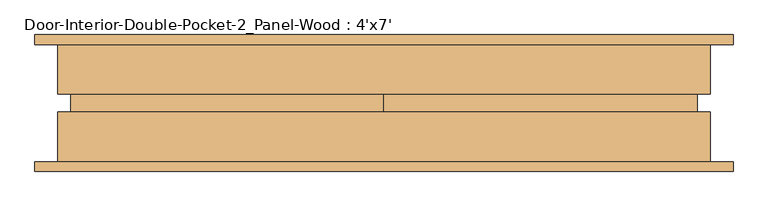
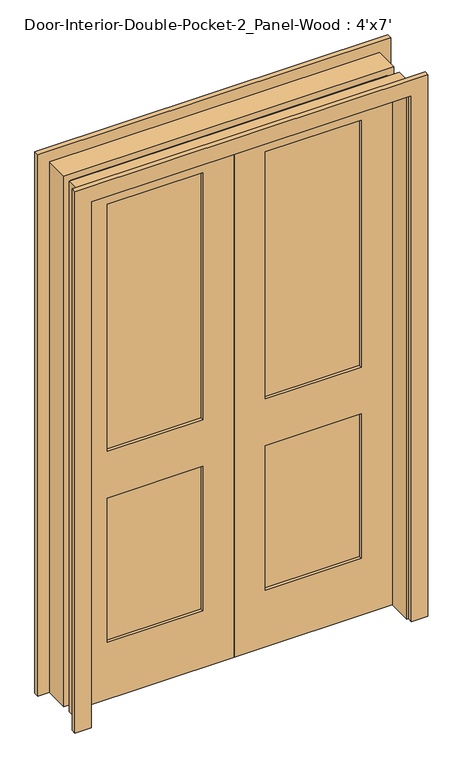
"""IFC4 building model written with IfcOpenShell, lengths in millimetres: door geometry, Door-Interior-Double-Pocket-2_Panel-Wood : 4'x7'."""

from ifc_helpers import new_model, si_unit, frame, origin, place, context, project, spatial, polyline, outline, extrude, source, transform, mapped, element, save


def door_interior_double_pocket_2_panel_wood_4_x7_3a565322(model_context):
    return source(origin(), model_context, "Body", "SweptSolid", [
        extrude(outline(polyline([(0.0, 615.95), (0.0, 679.45), (2203.45, 679.45), (2203.45, -679.45), (0.0, -679.45), (0.0, -615.95), (2139.95, -615.95), (2139.95, 615.95), (0.0, 615.95)])), frame((0.0, 114.3, 0.0), z_axis=(0.0, 1.0, 0.0), x_axis=(0.0, 0.0, 1.0)), (0.0, 0.0, 1.0), 19.05),
        extrude(outline(polyline([(0.0, 615.95), (0.0, 679.45), (2203.45, 679.45), (2203.45, -679.45), (0.0, -679.45), (0.0, -615.95), (2139.95, -615.95), (2139.95, 615.95), (0.0, 615.95)])), frame((0.0, -133.35, 0.0), z_axis=(0.0, 1.0, 0.0), x_axis=(0.0, 0.0, 1.0)), (0.0, 0.0, 1.0), 19.05),
        extrude(outline(polyline([(2133.6, 0.0), (0.0, 0.0), (0.0, 609.6), (2133.6, 609.6), (2133.6, 0.0)]), holes=[polyline([(2014.5375, 120.65), (2014.5375, 488.95), (1009.65, 488.95), (1009.65, 120.65), (2014.5375, 120.65)]), polyline([(819.15, 120.65), (819.15, 488.95), (231.775, 488.95), (231.775, 120.65), (819.15, 120.65)])]), frame((0.0, -17.4625, 0.0), z_axis=(0.0, 1.0, 0.0), x_axis=(0.0, 0.0, 1.0)), (0.0, 0.0, 1.0), 34.925),
        extrude(outline(polyline([(488.95, -5.8208333), (120.65, -5.8208333), (120.65, 5.8208333), (488.95, 5.8208333), (488.95, -5.8208333)])), frame((0.0, 0.0, 1009.65), z_axis=(0.0, 0.0, 1.0), x_axis=(1.0, 0.0, 0.0)), (0.0, 0.0, 1.0), 1004.8875),
        extrude(outline(polyline([(488.95, -5.8208333), (120.65, -5.8208333), (120.65, 5.8208333), (488.95, 5.8208333), (488.95, -5.8208333)])), frame((0.0, 0.0, 231.775), z_axis=(0.0, 0.0, 1.0), x_axis=(1.0, 0.0, 0.0)), (0.0, 0.0, 1.0), 587.375),
        extrude(outline(polyline([(0.0, 635.0), (2159.0, 635.0), (2159.0, -635.0), (0.0, -635.0), (0.0, -609.6), (2133.6, -609.6), (2133.6, 609.6), (0.0, 609.6), (0.0, 635.0)])), frame((0.0, 17.4625, 0.0), z_axis=(0.0, 1.0, 0.0), x_axis=(0.0, 0.0, 1.0)), (0.0, 0.0, 1.0), 96.8375),
        extrude(outline(polyline([(0.0, 635.0), (2159.0, 635.0), (2159.0, -635.0), (0.0, -635.0), (0.0, -609.6), (2133.6, -609.6), (2133.6, 609.6), (0.0, 609.6), (0.0, 635.0)])), frame((0.0, -114.3, 0.0), z_axis=(0.0, 1.0, 0.0), x_axis=(0.0, 0.0, 1.0)), (0.0, 0.0, 1.0), 96.8375),
        extrude(outline(polyline([(2133.6, -609.6), (0.0, -609.6), (0.0, 0.0), (2133.6, 0.0), (2133.6, -609.6)]), holes=[polyline([(2014.5375, -488.95), (2014.5375, -120.65), (1009.65, -120.65), (1009.65, -488.95), (2014.5375, -488.95)]), polyline([(819.15, -488.95), (819.15, -120.65), (231.775, -120.65), (231.775, -488.95), (819.15, -488.95)])]), frame((0.0, -17.4625, 0.0), z_axis=(0.0, 1.0, 0.0), x_axis=(0.0, 0.0, 1.0)), (0.0, 0.0, 1.0), 34.925),
        extrude(outline(polyline([(-120.65, -5.8208333), (-488.95, -5.8208333), (-488.95, 5.8208333), (-120.65, 5.8208333), (-120.65, -5.8208333)])), frame((0.0, 0.0, 1009.65), z_axis=(0.0, 0.0, 1.0), x_axis=(1.0, 0.0, 0.0)), (0.0, 0.0, 1.0), 1004.8875),
        extrude(outline(polyline([(-120.65, -5.8208333), (-488.95, -5.8208333), (-488.95, 5.8208333), (-120.65, 5.8208333), (-120.65, -5.8208333)])), frame((0.0, 0.0, 231.775), z_axis=(0.0, 0.0, 1.0), x_axis=(1.0, 0.0, 0.0)), (0.0, 0.0, 1.0), 587.375),
    ])


if __name__ == "__main__":
    model = new_model("IFC4")
    model_context = context("Model", 3, world=origin())
    ifc_project = project(units=[si_unit("LENGTHUNIT", "METRE", prefix="MILLI")], contexts=[model_context])
    site = spatial("IfcSite", under=ifc_project)
    building = spatial("IfcBuilding", under=site)
    placement = place(None, origin())
    door_interior_double_pocket_2_panel_wood_4_x7_shape = door_interior_double_pocket_2_panel_wood_4_x7_3a565322(model_context)
    element("IfcDoor", 1, ObjectType="Door-Interior-Double-Pocket-2_Panel-Wood : 4'x7'", at=placement, inside=building, context=model_context, shape_type="MappedRepresentation", body=[
        mapped(door_interior_double_pocket_2_panel_wood_4_x7_shape, transform((0.0, 0.0, 0.0), x_axis=(1.0, 0.0, 0.0), y_axis=(0.0, 1.0, 0.0), z_axis=(0.0, 0.0, 1.0))),
    ])
    save(model, "model.ifc")

# Revit data of these elements
# Type "Door-Interior-Double-Pocket-2_Panel-Wood : 4'x7'"
#   Type Mark = "9"
#   Assembly Code = "C1020300"
#   Analytic Construction = "Wooden"
#   Top Rail = 0' - 4 11/16"
#   Thickness = 0' - 1 3/8"
#   Thermal Resistance (R) = 2.5876 (h·ft²·°F)/BTU
#   Stiles = 0' - 4 3/4"
#   Rough Width = 8' - 2"
#   Rough Height = 7' - 4 1/2"
#   Panel Width = 2' - 0"
#   Lock Rail = 0' - 7 1/2"
#   Location [instance default] = 2' - 1"
#   Height = 7' - 0"
#   Width = 4' - 0"
#   Heat Transfer Coefficient (U) = 0.3865 BTU/(h·ft²·°F)
#   Bottom Rail = 0' - 9 1/8"
#   Panel Open [instance default] = no
#   Trim Material = Cherry
#   Panel Material = Cherry
#   Frame Material = Cherry
#   Visual Light Transmittance = 0
#   Solar Heat Gain Coefficient = 0
#   Wall Closure = (empty or 0)
#   Function = (empty or 0)
# Element 1 (IfcDoor, "Door-Interior-Double-Pocket-2_Panel-Wood : 4'x7'")
#   Materials on its faces: "Cherry"
# Materials
#   "Cherry": class "Wood", colour RGB 226 177 128, transparency 0, Description = "Prunus Serotina", Cost = 0
